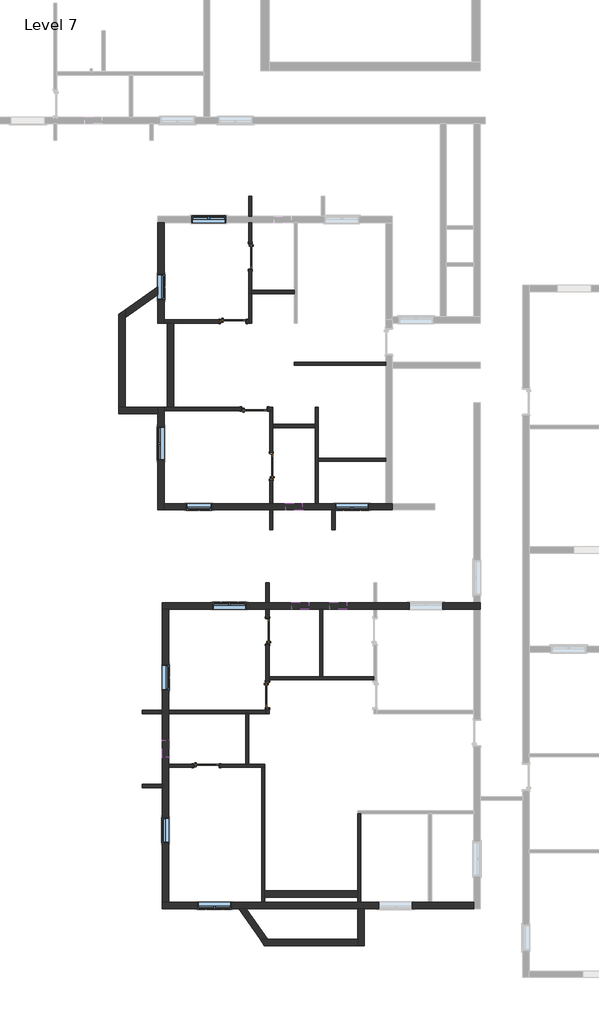
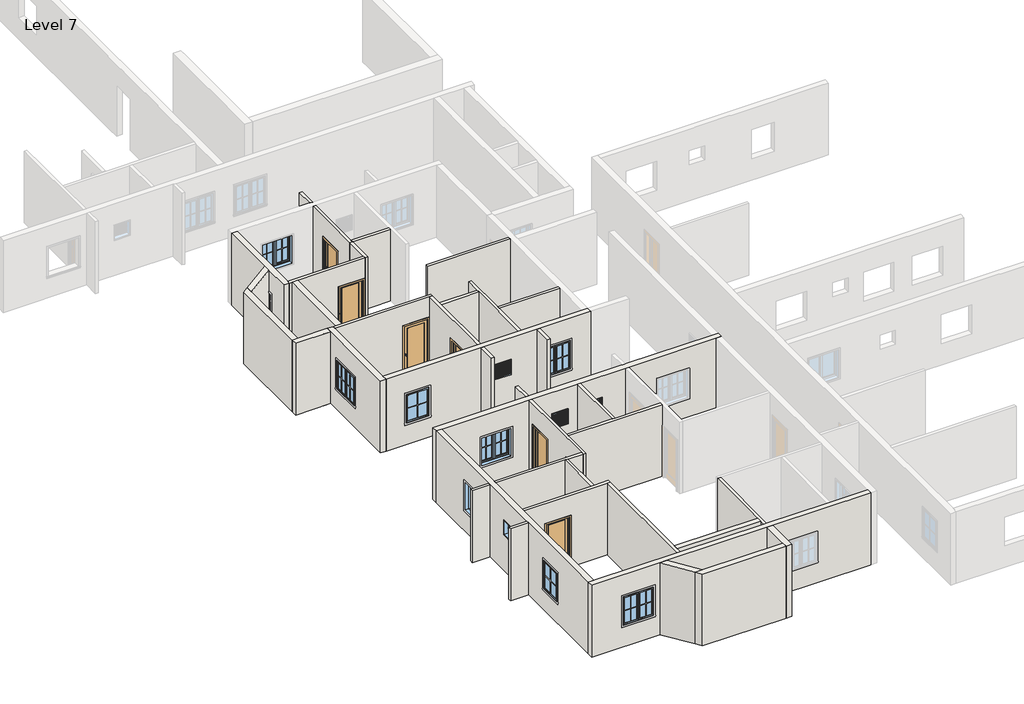
# One storey, part 1 of 7: 39 walls, 13 windows, 7 doors.
"""IFC4 building model written with IfcOpenShell, lengths in millimetres."""

from ifc_helpers import new_model, si_unit, frame, origin, place, context, project, spatial, polyline, outline, extrude, faceted_brep, transform, mapped, element, save
from components import door_3c6ab76a, door_a3feeac7, window_272f20d6, window_casement_double_4_x_4_af3140d2, window_f2d8fef0

model = new_model("IFC4")

# Units and contexts
model_context = context("Model", 3, world=origin())
ifc_project = project(units=[si_unit("LENGTHUNIT", "METRE", prefix="MILLI")], contexts=[model_context])

# Site, building, storey
site = spatial("IfcSite", under=ifc_project)
building = spatial("IfcBuilding", under=site)
storey = spatial("IfcBuildingStorey", under=building, Name="Level 7", Elevation=9601.2)

# Doors
placement = place(None, origin())
door_shape = door_3c6ab76a(model_context)
element("IfcDoor", 1, ObjectType="Door-Interior-Single-1_Panel-Wood : 2'6\" x 7' door", at=placement, inside=storey, context=model_context, shape_type="MappedRepresentation", body=[
    mapped(door_shape, transform((-4216.6759469, -3460.4538828, 9601.2), x_axis=(0.0, -1.0, 0.0), y_axis=(1.0, 0.0, 0.0), z_axis=(0.0, 0.0, 1.0))),
])
element("IfcDoor", 2, ObjectType="Door-Interior-Single-1_Panel-Wood : 2'6\" x 7' door", at=placement, inside=storey, context=model_context, shape_type="MappedRepresentation", body=[
    mapped(door_shape, transform((-5797.8259469, -21840.5288828, 9601.2), x_axis=(1.0, 0.0, 0.0), y_axis=(0.0, 1.0, 0.0), z_axis=(0.0, 0.0, 1.0))),
])
door_2_shape = door_a3feeac7(model_context)
element("IfcDoor", 3, ObjectType="Door-Interior-Single-1_Panel-Wood : 2'6\" x 7' door", at=placement, inside=storey, context=model_context, shape_type="MappedRepresentation", body=[
    mapped(door_2_shape, transform((-3454.6759469, -11032.8288828, 9601.2), x_axis=(0.0, 1.0, 0.0), y_axis=(-1.0, 0.0, 0.0), z_axis=(0.0, 0.0, 1.0))),
])
element("IfcDoor", 4, ObjectType="Door-Interior-Single-1_Panel-Wood : 2'6\" x 7' door", at=placement, inside=storey, context=model_context, shape_type="MappedRepresentation", body=[
    mapped(door_2_shape, transform((-3594.3759469, -16985.9538828, 9601.2), x_axis=(0.0, 1.0, 0.0), y_axis=(-1.0, 0.0, 0.0), z_axis=(0.0, 0.0, 1.0))),
])
element("IfcDoor", 5, ObjectType="Door-Interior-Single-1_Panel-Wood : 36\" x 84\"", at=placement, inside=storey, context=model_context, shape_type="MappedRepresentation", body=[
    mapped(door_shape, transform((-4829.4509469, -5800.4288828, 9601.2), x_axis=(1.0, 0.0, 0.0), y_axis=(0.0, 1.0, 0.0), z_axis=(0.0, 0.0, 1.0))),
])
element("IfcDoor", 6, ObjectType="Door-Interior-Single-1_Panel-Wood : 36\" x 84\"", at=placement, inside=storey, context=model_context, shape_type="MappedRepresentation", body=[
    mapped(door_2_shape, transform((-4067.4509469, -8969.0788828, 9601.2), x_axis=(1.0, 0.0, 0.0), y_axis=(0.0, 1.0, 0.0), z_axis=(0.0, 0.0, 1.0))),
])
element("IfcDoor", 7, ObjectType="Door-Interior-Single-1_Panel-Wood : 36\" x 84\"", at=placement, inside=storey, context=model_context, shape_type="MappedRepresentation", body=[
    mapped(door_2_shape, transform((-3600.7259469, -19291.0038828, 9601.2), x_axis=(0.0, -1.0, 0.0), y_axis=(1.0, 0.0, 0.0), z_axis=(0.0, 0.0, 1.0))),
])

# Walls
element("IfcWall", 8, ObjectType="4.5\" wall", at=placement, inside=storey, context=model_context, shape_type="Brep", body=[
    faceted_brep([(-4277.0009469, -4793.9538828, 12649.2), (-4277.0009469, -2241.2538828, 12649.2), (-4277.0009469, -2241.2538828, 9601.2), (-4277.0009469, -2977.8538828, 9601.2), (-4277.0009469, -2977.8538828, 11760.2), (-4277.0009469, -3943.0538828, 11760.2), (-4277.0009469, -3943.0538828, 9601.2), (-4277.0009469, -4793.9538828, 9601.2), (-4162.7009469, -2241.2538828, 12649.2), (-4162.7009469, -4679.6538828, 12649.2), (-4162.7009469, -4793.9538828, 12649.2), (-4162.7009469, -4793.9538828, 9601.2), (-4162.7009469, -4679.6538828, 9601.2), (-4162.7009469, -3943.0538828, 9601.2), (-4162.7009469, -3943.0538828, 11760.2), (-4162.7009469, -2977.8538828, 11760.2), (-4162.7009469, -2977.8538828, 9601.2), (-4162.7009469, -2241.2538828, 9601.2)], [[[0, 1, 2, 3, 4, 5, 6, 7]], [[8, 9, 10, 11, 12, 13, 14, 15, 16, 17]], [[2, 17, 16, 3]], [[11, 7, 6, 13, 12]], [[1, 0, 10, 9, 8]], [[2, 1, 8, 17]], [[0, 7, 11, 10]], [[5, 14, 13, 6]], [[14, 5, 4, 15]], [[15, 4, 3, 16]]]),
])
element("IfcWall", 9, ObjectType="4.5\" wall", at=placement, inside=storey, context=model_context, shape_type="Brep", body=[
    faceted_brep([(-4277.0009469, -4793.9538828, 9601.2), (-4277.0009469, -5746.4538828, 9601.2), (-4277.0009469, -5860.7538828, 9601.2), (-4277.0009469, -5860.7538828, 12649.2), (-4277.0009469, -5746.4538828, 12649.2), (-4277.0009469, -4793.9538828, 12649.2), (-4162.7009469, -4793.9538828, 9601.2), (-4162.7009469, -4793.9538828, 12649.2), (-4162.7009469, -5860.7538828, 12649.2), (-4162.7009469, -5860.7538828, 9601.2)], [[[0, 1, 2, 3, 4, 5]], [[6, 7, 8, 9]], [[2, 1, 0, 6, 9]], [[5, 4, 3, 8, 7]], [[0, 5, 7, 6]], [[3, 2, 9, 8]]]),
])
element("IfcWall", 10, ObjectType="4.5\" wall", at=placement, inside=storey, context=model_context, shape_type="Brep", body=[
    faceted_brep([(-7325.0009469, -5746.4538828, 12649.2), (-4277.0009469, -5746.4538828, 12649.2), (-4277.0009469, -5746.4538828, 9601.2), (-4346.8509469, -5746.4538828, 9601.2), (-4346.8509469, -5746.4538828, 11760.2), (-5312.0509469, -5746.4538828, 11760.2), (-5312.0509469, -5746.4538828, 9601.2), (-7325.0009469, -5746.4538828, 9601.2), (-4277.0009469, -5860.7538828, 12649.2), (-6982.1009469, -5860.7538828, 12649.2), (-7210.7009469, -5860.7538828, 12649.2), (-7325.0009469, -5860.7538828, 12649.2), (-7325.0009469, -5860.7538828, 9601.2), (-7210.7009469, -5860.7538828, 9601.2), (-6982.1009469, -5860.7538828, 9601.2), (-5312.0509469, -5860.7538828, 9601.2), (-5312.0509469, -5860.7538828, 11760.2), (-4346.8509469, -5860.7538828, 11760.2), (-4346.8509469, -5860.7538828, 9601.2), (-4277.0009469, -5860.7538828, 9601.2)], [[[0, 1, 2, 3, 4, 5, 6, 7]], [[8, 9, 10, 11, 12, 13, 14, 15, 16, 17, 18, 19]], [[12, 7, 6, 15, 14, 13]], [[2, 19, 18, 3]], [[1, 0, 11, 10, 9, 8]], [[0, 7, 12, 11]], [[2, 1, 8, 19]], [[17, 4, 3, 18]], [[4, 17, 16, 5]], [[5, 16, 15, 6]]]),
])
element("IfcWall", 11, ObjectType="4.5\" wall", at=placement, inside=storey, context=model_context, shape_type="SweptSolid", body=[
    extrude(outline(polyline([(-2638.7009469, -4793.9538828), (-4162.7009469, -4793.9538828), (-4162.7009469, -4679.6538828), (-2638.7009469, -4679.6538828), (-2638.7009469, -4793.9538828)])), frame((0.0, 0.0, 9601.2), z_axis=(0.0, 0.0, 1.0), x_axis=(1.0, 0.0, 0.0)), (0.0, 0.0, 1.0), 3048.0),
])
element("IfcWall", 12, ObjectType="4.5\" wall", at=placement, inside=storey, context=model_context, shape_type="SweptSolid", body=[
    extrude(outline(polyline([(-2638.7009469, -7270.4538828), (675.9990531, -7270.4538828), (675.9990531, -7384.7538828), (-2638.7009469, -7384.7538828), (-2638.7009469, -7270.4538828)])), frame((0.0, 0.0, 9601.2), z_axis=(0.0, 0.0, 1.0), x_axis=(1.0, 0.0, 0.0)), (0.0, 0.0, 1.0), 3048.0),
])
element("IfcWall", 13, ObjectType="4.5\" wall", at=placement, inside=storey, context=model_context, shape_type="Brep", body=[
    faceted_brep([(-7325.0009469, -8908.7538828, 12649.2), (-7210.7009469, -8908.7538828, 12649.2), (-6982.1009469, -8908.7538828, 12649.2), (-3400.7009469, -8908.7538828, 12649.2), (-3400.7009469, -8908.7538828, 9601.2), (-3584.8509469, -8908.7538828, 9601.2), (-3584.8509469, -8908.7538828, 11760.2), (-4550.0509469, -8908.7538828, 11760.2), (-4550.0509469, -8908.7538828, 9601.2), (-6982.1009469, -8908.7538828, 9601.2), (-7210.7009469, -8908.7538828, 9601.2), (-7325.0009469, -8908.7538828, 9601.2), (-3400.7009469, -9023.0538828, 12649.2), (-3515.0009469, -9023.0538828, 12649.2), (-7325.0009469, -9023.0538828, 12649.2), (-7325.0009469, -9023.0538828, 9601.2), (-4550.0509469, -9023.0538828, 9601.2), (-4550.0509469, -9023.0538828, 11760.2), (-3584.8509469, -9023.0538828, 11760.2), (-3584.8509469, -9023.0538828, 9601.2), (-3515.0009469, -9023.0538828, 9601.2), (-3400.7009469, -9023.0538828, 9601.2)], [[[0, 1, 2, 3, 4, 5, 6, 7, 8, 9, 10, 11]], [[12, 13, 14, 15, 16, 17, 18, 19, 20, 21]], [[4, 21, 20, 19, 5]], [[15, 11, 10, 9, 8, 16]], [[3, 2, 1, 0, 14, 13, 12]], [[4, 3, 12, 21]], [[0, 11, 15, 14]], [[18, 6, 5, 19]], [[6, 18, 17, 7]], [[7, 17, 16, 8]]]),
])
element("IfcWall", 14, ObjectType="4.5\" wall", at=placement, inside=storey, context=model_context, shape_type="SweptSolid", body=[
    extrude(outline(polyline([(-1876.7009469, -9632.6538828), (-3400.7009469, -9632.6538828), (-3400.7009469, -9518.3538828), (-1876.7009469, -9518.3538828), (-1876.7009469, -9632.6538828)])), frame((0.0, 0.0, 9601.2), z_axis=(0.0, 0.0, 1.0), x_axis=(1.0, 0.0, 0.0)), (0.0, 0.0, 1.0), 3048.0),
])
element("IfcWall", 15, ObjectType="4.5\" wall", at=placement, inside=storey, context=model_context, shape_type="Brep", body=[
    faceted_brep([(-1762.4009469, -12375.8538828, 9601.2), (-1762.4009469, -10851.8538828, 9601.2), (-1762.4009469, -10737.5538828, 9601.2), (-1762.4009469, -8908.7538828, 9601.2), (-1762.4009469, -8908.7538828, 12649.2), (-1762.4009469, -10737.5538828, 12649.2), (-1762.4009469, -10851.8538828, 12649.2), (-1762.4009469, -12375.8538828, 12649.2), (-1876.7009469, -12375.8538828, 9601.2), (-1876.7009469, -12375.8538828, 12649.2), (-1876.7009469, -9632.6538828, 12649.2), (-1876.7009469, -9518.3538828, 12649.2), (-1876.7009469, -8908.7538828, 12649.2), (-1876.7009469, -8908.7538828, 9601.2), (-1876.7009469, -9518.3538828, 9601.2), (-1876.7009469, -9632.6538828, 9601.2)], [[[0, 1, 2, 3, 4, 5, 6, 7]], [[8, 9, 10, 11, 12, 13, 14, 15]], [[3, 2, 1, 0, 8, 15, 14, 13]], [[4, 3, 13, 12]], [[7, 6, 5, 4, 12, 11, 10, 9]], [[0, 7, 9, 8]]]),
])
element("IfcWall", 16, ObjectType="4.5\" wall", at=placement, inside=storey, context=model_context, shape_type="Brep", body=[
    faceted_brep([(-3400.7009469, -9023.0538828, 12649.2), (-3400.7009469, -9518.3538828, 12649.2), (-3400.7009469, -9632.6538828, 12649.2), (-3400.7009469, -12375.8538828, 12649.2), (-3400.7009469, -12375.8538828, 9601.2), (-3400.7009469, -11515.4288828, 9601.2), (-3400.7009469, -11515.4288828, 11760.2), (-3400.7009469, -10550.2288828, 11760.2), (-3400.7009469, -10550.2288828, 9601.2), (-3400.7009469, -9632.6538828, 9601.2), (-3400.7009469, -9518.3538828, 9601.2), (-3400.7009469, -9023.0538828, 9601.2), (-3515.0009469, -12375.8538828, 12649.2), (-3515.0009469, -9023.0538828, 12649.2), (-3515.0009469, -9023.0538828, 9601.2), (-3515.0009469, -10550.2288828, 9601.2), (-3515.0009469, -10550.2288828, 11760.2), (-3515.0009469, -11515.4288828, 11760.2), (-3515.0009469, -11515.4288828, 9601.2), (-3515.0009469, -12375.8538828, 9601.2)], [[[0, 1, 2, 3, 4, 5, 6, 7, 8, 9, 10, 11]], [[12, 13, 14, 15, 16, 17, 18, 19]], [[4, 19, 18, 5]], [[14, 11, 10, 9, 8, 15]], [[3, 2, 1, 0, 13, 12]], [[4, 3, 12, 19]], [[0, 11, 14, 13]], [[7, 16, 15, 8]], [[16, 7, 6, 17]], [[17, 6, 5, 18]]]),
])
element("IfcWall", 17, ObjectType="4.5\" wall", at=placement, inside=storey, context=model_context, shape_type="SweptSolid", body=[
    extrude(outline(polyline([(-1762.4009469, -10737.5538828), (675.9990531, -10737.5538828), (675.9990531, -10851.8538828), (-1762.4009469, -10851.8538828), (-1762.4009469, -10737.5538828)])), frame((0.0, 0.0, 9601.2), z_axis=(0.0, 0.0, 1.0), x_axis=(1.0, 0.0, 0.0)), (0.0, 0.0, 1.0), 3048.0),
])
element("IfcWall", 18, ObjectType="4.5\" wall", at=placement, inside=storey, context=model_context, shape_type="SweptSolid", body=[
    extrude(outline(polyline([(-3515.0009469, -13328.3538828), (-3515.0009469, -12604.4538828), (-3400.7009469, -12604.4538828), (-3400.7009469, -13328.3538828), (-3515.0009469, -13328.3538828)])), frame((0.0, 0.0, 9601.2), z_axis=(0.0, 0.0, 1.0), x_axis=(1.0, 0.0, 0.0)), (0.0, 0.0, 1.0), 3048.0),
])
element("IfcWall", 19, ObjectType="4.5\" wall", at=placement, inside=storey, context=model_context, shape_type="Brep", body=[
    faceted_brep([(-1152.8009469, -13328.3538828, 9601.2), (-1152.8009469, -12604.4538828, 9601.2), (-1152.8009469, -12604.4538828, 10515.6), (-1152.8009469, -12604.4538828, 11734.8), (-1152.8009469, -12604.4538828, 12649.2), (-1152.8009469, -13328.3538828, 12649.2), (-1267.1009469, -13328.3538828, 9601.2), (-1267.1009469, -13328.3538828, 12649.2), (-1267.1009469, -12604.4538828, 12649.2), (-1267.1009469, -12604.4538828, 9601.2)], [[[0, 1, 2, 3, 4, 5]], [[6, 7, 8, 9]], [[1, 0, 6, 9]], [[5, 4, 8, 7]], [[0, 5, 7, 6]], [[4, 3, 2, 1, 9, 8]]]),
])
element("IfcWall", 20, ObjectType="4.5\" wall", at=placement, inside=storey, context=model_context, shape_type="SweptSolid", body=[
    extrude(outline(polyline([(-4162.7009469, -1288.7538828), (-4162.7009469, -2012.6538828), (-4277.0009469, -2012.6538828), (-4277.0009469, -1288.7538828), (-4162.7009469, -1288.7538828)])), frame((0.0, 0.0, 9601.2), z_axis=(0.0, 0.0, 1.0), x_axis=(1.0, 0.0, 0.0)), (0.0, 0.0, 1.0), 3048.0),
])
element("IfcWall", 21, ObjectType="4.5\" wall", at=placement, inside=storey, context=model_context, shape_type="Brep", body=[
    faceted_brep([(231.4990531, -18624.2538828, 9601.2), (-1597.3009469, -18624.2538828, 9601.2), (-1711.6009469, -18624.2538828, 9601.2), (-3540.4009469, -18624.2538828, 9601.2), (-3540.4009469, -18624.2538828, 12649.2), (-1711.6009469, -18624.2538828, 12649.2), (-1597.3009469, -18624.2538828, 12649.2), (231.4990531, -18624.2538828, 12649.2), (231.4990531, -18738.5538828, 9601.2), (231.4990531, -18738.5538828, 12649.2), (-3540.4009469, -18738.5538828, 12649.2), (-3540.4009469, -18738.5538828, 9601.2)], [[[0, 1, 2, 3, 4, 5, 6, 7]], [[8, 9, 10, 11]], [[3, 2, 1, 0, 8, 11]], [[7, 6, 5, 4, 10, 9]], [[4, 3, 11, 10]], [[0, 7, 9, 8]]]),
])
element("IfcWall", 22, ObjectType="4.5\" wall", at=placement, inside=storey, context=model_context, shape_type="SweptSolid", body=[
    extrude(outline(polyline([(-1597.3009469, -16185.8538828), (-1597.3009469, -18624.2538828), (-1711.6009469, -18624.2538828), (-1711.6009469, -16185.8538828), (-1597.3009469, -16185.8538828)])), frame((0.0, 0.0, 9601.2), z_axis=(0.0, 0.0, 1.0), x_axis=(1.0, 0.0, 0.0)), (0.0, 0.0, 1.0), 3048.0),
])
element("IfcWall", 23, ObjectType="4.5\" wall", at=placement, inside=storey, context=model_context, shape_type="SweptSolid", body=[
    extrude(outline(polyline([(-3540.4009469, -15233.3538828), (-3540.4009469, -15957.2538828), (-3654.7009469, -15957.2538828), (-3654.7009469, -15233.3538828), (-3540.4009469, -15233.3538828)])), frame((0.0, 0.0, 9601.2), z_axis=(0.0, 0.0, 1.0), x_axis=(1.0, 0.0, 0.0)), (0.0, 0.0, 1.0), 3048.0),
])
element("IfcWall", 24, ObjectType="4.5\" wall", at=placement, inside=storey, context=model_context, shape_type="Brep", body=[
    faceted_brep([(-3654.7009469, -19957.7538828, 12649.2), (-3654.7009469, -19843.4538828, 12649.2), (-3654.7009469, -16185.8538828, 12649.2), (-3654.7009469, -16185.8538828, 9601.2), (-3654.7009469, -16503.3538828, 9601.2), (-3654.7009469, -16503.3538828, 11760.2), (-3654.7009469, -17468.5538828, 11760.2), (-3654.7009469, -17468.5538828, 9601.2), (-3654.7009469, -18808.4038828, 9601.2), (-3654.7009469, -18808.4038828, 11760.2), (-3654.7009469, -19773.6038828, 11760.2), (-3654.7009469, -19773.6038828, 9601.2), (-3654.7009469, -19843.4538828, 9601.2), (-3654.7009469, -19957.7538828, 9601.2), (-3540.4009469, -16185.8538828, 12649.2), (-3540.4009469, -18624.2538828, 12649.2), (-3540.4009469, -18738.5538828, 12649.2), (-3540.4009469, -19957.7538828, 12649.2), (-3540.4009469, -19957.7538828, 9601.2), (-3540.4009469, -19773.6038828, 9601.2), (-3540.4009469, -19773.6038828, 11760.2), (-3540.4009469, -18808.4038828, 11760.2), (-3540.4009469, -18808.4038828, 9601.2), (-3540.4009469, -18738.5538828, 9601.2), (-3540.4009469, -18624.2538828, 9601.2), (-3540.4009469, -17468.5538828, 9601.2), (-3540.4009469, -17468.5538828, 11760.2), (-3540.4009469, -16503.3538828, 11760.2), (-3540.4009469, -16503.3538828, 9601.2), (-3540.4009469, -16185.8538828, 9601.2)], [[[0, 1, 2, 3, 4, 5, 6, 7, 8, 9, 10, 11, 12, 13]], [[14, 15, 16, 17, 18, 19, 20, 21, 22, 23, 24, 25, 26, 27, 28, 29]], [[3, 29, 28, 4]], [[18, 13, 12, 11, 19]], [[7, 25, 24, 23, 22, 8]], [[2, 1, 0, 17, 16, 15, 14]], [[3, 2, 14, 29]], [[0, 13, 18, 17]], [[27, 5, 4, 28]], [[5, 27, 26, 6]], [[6, 26, 25, 7]], [[10, 20, 19, 11]], [[20, 10, 9, 21]], [[21, 9, 8, 22]]]),
])
element("IfcWall", 25, ObjectType="4.5\" wall", at=placement, inside=storey, context=model_context, shape_type="Brep", body=[
    faceted_brep([(-3654.7009469, -19843.4538828, 9601.2), (-7159.9009469, -19843.4538828, 9601.2), (-7159.9009469, -19843.4538828, 12649.2), (-3654.7009469, -19843.4538828, 12649.2), (-3654.7009469, -19957.7538828, 9601.2), (-3654.7009469, -19957.7538828, 12649.2), (-4264.3009469, -19957.7538828, 12649.2), (-4378.6009469, -19957.7538828, 12649.2), (-7159.9009469, -19957.7538828, 12649.2), (-7159.9009469, -19957.7538828, 9601.2), (-4378.6009469, -19957.7538828, 9601.2), (-4264.3009469, -19957.7538828, 9601.2)], [[[0, 1, 2, 3]], [[4, 5, 6, 7, 8, 9, 10, 11]], [[1, 0, 4, 11, 10, 9]], [[3, 2, 8, 7, 6, 5]], [[2, 1, 9, 8]], [[0, 3, 5, 4]]]),
])
element("IfcWall", 26, ObjectType="4.5\" wall", at=placement, inside=storey, context=model_context, shape_type="Brep", body=[
    faceted_brep([(-7159.9009469, -21786.5538828, 12649.2), (-4378.6009469, -21786.5538828, 12649.2), (-4264.3009469, -21786.5538828, 12649.2), (-3692.8009469, -21786.5538828, 12649.2), (-3692.8009469, -21786.5538828, 9601.2), (-4264.3009469, -21786.5538828, 9601.2), (-4378.6009469, -21786.5538828, 9601.2), (-5315.2259469, -21786.5538828, 9601.2), (-5315.2259469, -21786.5538828, 11760.2), (-6280.4259469, -21786.5538828, 11760.2), (-6280.4259469, -21786.5538828, 9601.2), (-7159.9009469, -21786.5538828, 9601.2), (-3692.8009469, -21900.8538828, 12649.2), (-3807.1009469, -21900.8538828, 12649.2), (-7159.9009469, -21900.8538828, 12649.2), (-7159.9009469, -21900.8538828, 9601.2), (-6280.4259469, -21900.8538828, 9601.2), (-6280.4259469, -21900.8538828, 11760.2), (-5315.2259469, -21900.8538828, 11760.2), (-5315.2259469, -21900.8538828, 9601.2), (-3807.1009469, -21900.8538828, 9601.2), (-3692.8009469, -21900.8538828, 9601.2)], [[[0, 1, 2, 3, 4, 5, 6, 7, 8, 9, 10, 11]], [[12, 13, 14, 15, 16, 17, 18, 19, 20, 21]], [[15, 11, 10, 16]], [[4, 21, 20, 19, 7, 6, 5]], [[3, 2, 1, 0, 14, 13, 12]], [[0, 11, 15, 14]], [[4, 3, 12, 21]], [[18, 8, 7, 19]], [[8, 18, 17, 9]], [[9, 17, 16, 10]]]),
])
element("IfcWall", 27, ObjectType="4.5\" wall", at=placement, inside=storey, context=model_context, shape_type="Brep", body=[
    faceted_brep([(-3692.8009469, -26777.6538828, 9601.2), (-3692.8009469, -26587.1538828, 9601.2), (-3692.8009469, -26358.5538828, 9601.2), (-3692.8009469, -21900.8538828, 9601.2), (-3692.8009469, -21900.8538828, 12649.2), (-3692.8009469, -26358.5538828, 12649.2), (-3692.8009469, -26587.1538828, 12649.2), (-3692.8009469, -26777.6538828, 12649.2), (-3807.1009469, -26777.6538828, 9601.2), (-3807.1009469, -26777.6538828, 12649.2), (-3807.1009469, -21900.8538828, 12649.2), (-3807.1009469, -21900.8538828, 9601.2)], [[[0, 1, 2, 3, 4, 5, 6, 7]], [[8, 9, 10, 11]], [[3, 2, 1, 0, 8, 11]], [[7, 6, 5, 4, 10, 9]], [[4, 3, 11, 10]], [[0, 7, 9, 8]]]),
])
element("IfcWall", 28, ObjectType="4.5\" wall", at=placement, inside=storey, context=model_context, shape_type="SweptSolid", body=[
    extrude(outline(polyline([(-7388.5009469, -22629.8863256), (-8112.4009469, -22629.8863256), (-8112.4009469, -22515.5863256), (-7388.5009469, -22515.5863256), (-7388.5009469, -22629.8863256)])), frame((0.0, 0.0, 9601.2), z_axis=(0.0, 0.0, 1.0), x_axis=(1.0, 0.0, 0.0)), (0.0, 0.0, 1.0), 3048.0),
])
element("IfcWall", 29, ObjectType="4.5\" wall", at=placement, inside=storey, context=model_context, shape_type="SweptSolid", body=[
    extrude(outline(polyline([(-8112.4009469, -19843.4538828), (-7388.5009469, -19843.4538828), (-7388.5009469, -19957.7538828), (-8112.4009469, -19957.7538828), (-8112.4009469, -19843.4538828)])), frame((0.0, 0.0, 9601.2), z_axis=(0.0, 0.0, 1.0), x_axis=(1.0, 0.0, 0.0)), (0.0, 0.0, 1.0), 3048.0),
])
element("IfcWall", 30, ObjectType="4.5\" wall", at=placement, inside=storey, context=model_context, shape_type="SweptSolid", body=[
    extrude(outline(polyline([(-4378.6009469, -21786.5538828), (-4378.6009469, -19957.7538828), (-4264.3009469, -19957.7538828), (-4264.3009469, -21786.5538828), (-4378.6009469, -21786.5538828)])), frame((0.0, 0.0, 9601.2), z_axis=(0.0, 0.0, 1.0), x_axis=(1.0, 0.0, 0.0)), (0.0, 0.0, 1.0), 3048.0),
])
element("IfcWall", 31, ObjectType="4.5\" wall", at=placement, inside=storey, context=model_context, shape_type="Brep", body=[
    faceted_brep([(-340.0009469, -23577.2538828, 9601.2), (-340.0009469, -26358.5538828, 9601.2), (-340.0009469, -26587.1538828, 9601.2), (-340.0009469, -26777.6538828, 9601.2), (-340.0009469, -26777.6538828, 12649.2), (-340.0009469, -26587.1538828, 12649.2), (-340.0009469, -26358.5538828, 12649.2), (-340.0009469, -23577.2538828, 12649.2), (-225.7009469, -23577.2538828, 9601.2), (-225.7009469, -23577.2538828, 12649.2), (-225.7009469, -26777.6538828, 12649.2), (-225.7009469, -26777.6538828, 9601.2)], [[[0, 1, 2, 3, 4, 5, 6, 7]], [[8, 9, 10, 11]], [[3, 2, 1, 0, 8, 11]], [[7, 6, 5, 4, 10, 9]], [[0, 7, 9, 8]], [[4, 3, 11, 10]]]),
])
element("IfcWall", 32, ObjectType="9\"", at=placement, inside=storey, context=model_context, shape_type="Brep", body=[
    faceted_brep([(-7553.6009469, -2241.2538828, 9601.2), (-7553.6009469, -4556.8220214, 9601.2), (-7553.6009469, -4835.8638828, 9601.2), (-7553.6009469, -5860.7538828, 9601.2), (-7553.6009469, -5860.7538828, 12649.2), (-7553.6009469, -4835.8638828, 12649.2), (-7553.6009469, -4556.8220214, 12649.2), (-7553.6009469, -2241.2538828, 12649.2), (-7553.6009469, -5016.2038828, 11734.8), (-7553.6009469, -5016.2038828, 10515.6), (-7553.6009469, -4101.8038828, 10515.6), (-7553.6009469, -4101.8038828, 11734.8), (-7325.0009469, -2241.2538828, 9601.2), (-7325.0009469, -2241.2538828, 12649.2), (-7325.0009469, -5746.4538828, 12649.2), (-7325.0009469, -5860.7538828, 12649.2), (-7325.0009469, -5860.7538828, 9601.2), (-7325.0009469, -5746.4538828, 9601.2), (-7325.0009469, -5016.2038828, 11734.8), (-7325.0009469, -4101.8038828, 11734.8), (-7325.0009469, -4101.8038828, 10515.6), (-7325.0009469, -5016.2038828, 10515.6)], [[[0, 1, 2, 3, 4, 5, 6, 7], [8, 9, 10, 11]], [[12, 13, 14, 15, 16, 17], [18, 19, 20, 21]], [[3, 2, 1, 0, 12, 17, 16]], [[7, 6, 5, 4, 15, 14, 13]], [[0, 7, 13, 12]], [[4, 3, 16, 15]], [[9, 8, 18, 21]], [[10, 9, 21, 20]], [[11, 10, 20, 19]], [[8, 11, 19, 18]]]),
])
element("IfcWall", 33, ObjectType="9\"", at=placement, inside=storey, context=model_context, shape_type="SweptSolid", body=[
    extrude(outline(polyline([(-6982.1009469, -5860.7538828), (-6982.1009469, -8908.7538828), (-7210.7009469, -8908.7538828), (-7210.7009469, -5860.7538828), (-6982.1009469, -5860.7538828)])), frame((0.0, 0.0, 9601.2), z_axis=(0.0, 0.0, 1.0), x_axis=(1.0, 0.0, 0.0)), (0.0, 0.0, 1.0), 3048.0),
])
element("IfcWall", 34, ObjectType="9\"", at=placement, inside=storey, context=model_context, shape_type="Brep", body=[
    faceted_brep([(-7553.6009469, -8908.7538828, 9601.2), (-7553.6009469, -9137.3538828, 9601.2), (-7553.6009469, -12604.4538828, 9601.2), (-7553.6009469, -12604.4538828, 12649.2), (-7553.6009469, -9137.3538828, 12649.2), (-7553.6009469, -8908.7538828, 12649.2), (-7553.6009469, -9600.9038828, 11734.8), (-7553.6009469, -10820.1038828, 11734.8), (-7553.6009469, -10820.1038828, 10515.6), (-7553.6009469, -9600.9038828, 10515.6), (-7325.0009469, -8908.7538828, 9601.2), (-7325.0009469, -8908.7538828, 12649.2), (-7325.0009469, -9023.0538828, 12649.2), (-7325.0009469, -12375.8538828, 12649.2), (-7325.0009469, -12604.4538828, 12649.2), (-7325.0009469, -12604.4538828, 9601.2), (-7325.0009469, -12375.8538828, 9601.2), (-7325.0009469, -9023.0538828, 9601.2), (-7325.0009469, -9600.9038828, 11734.8), (-7325.0009469, -9600.9038828, 10515.6), (-7325.0009469, -10820.1038828, 10515.6), (-7325.0009469, -10820.1038828, 11734.8)], [[[0, 1, 2, 3, 4, 5], [6, 7, 8, 9]], [[10, 11, 12, 13, 14, 15, 16, 17], [18, 19, 20, 21]], [[2, 1, 0, 10, 17, 16, 15]], [[5, 4, 3, 14, 13, 12, 11]], [[3, 2, 15, 14]], [[0, 5, 11, 10]], [[19, 18, 6, 9]], [[20, 19, 9, 8]], [[21, 20, 8, 7]], [[18, 21, 7, 6]]]),
])
element("IfcWall", 35, ObjectType="9\"", at=placement, inside=storey, context=model_context, shape_type="Brep", body=[
    faceted_brep([(-7325.0009469, -12604.4538828, 9601.2), (-3515.0009469, -12604.4538828, 9601.2), (-3400.7009469, -12604.4538828, 9601.2), (-1267.1009469, -12604.4538828, 9601.2), (-1152.8009469, -12604.4538828, 9601.2), (904.5990531, -12604.4538828, 9601.2), (904.5990531, -12604.4538828, 12649.2), (-1152.8009469, -12604.4538828, 12649.2), (-1267.1009469, -12604.4538828, 12649.2), (-3400.7009469, -12604.4538828, 12649.2), (-3515.0009469, -12604.4538828, 12649.2), (-7325.0009469, -12604.4538828, 12649.2), (-2333.9009469, -12604.4538828, 11734.8), (-2333.9009469, -12604.4538828, 11125.2), (-2943.5009469, -12604.4538828, 11125.2), (-2943.5009469, -12604.4538828, 11734.8), (-6524.9009469, -12604.4538828, 11734.8), (-5610.5009469, -12604.4538828, 11734.8), (-5610.5009469, -12604.4538828, 10515.6), (-6524.9009469, -12604.4538828, 10515.6), (-1152.8009469, -12604.4538828, 11734.8), (66.3990531, -12604.4538828, 11734.8), (66.3990531, -12604.4538828, 10515.6), (-1152.8009469, -12604.4538828, 10515.6), (-7325.0009469, -12375.8538828, 9601.2), (-7325.0009469, -12375.8538828, 12649.2), (-3515.0009469, -12375.8538828, 12649.2), (-3400.7009469, -12375.8538828, 12649.2), (-1876.7009469, -12375.8538828, 12649.2), (-1762.4009469, -12375.8538828, 12649.2), (675.9990531, -12375.8538828, 12649.2), (904.5990531, -12375.8538828, 12649.2), (904.5990531, -12375.8538828, 9601.2), (675.9990531, -12375.8538828, 9601.2), (-1762.4009469, -12375.8538828, 9601.2), (-1876.7009469, -12375.8538828, 9601.2), (-3400.7009469, -12375.8538828, 9601.2), (-3515.0009469, -12375.8538828, 9601.2), (-2333.9009469, -12375.8538828, 11734.8), (-2943.5009469, -12375.8538828, 11734.8), (-2943.5009469, -12375.8538828, 11125.2), (-2333.9009469, -12375.8538828, 11125.2), (-6524.9009469, -12375.8538828, 11734.8), (-6524.9009469, -12375.8538828, 10515.6), (-5610.5009469, -12375.8538828, 10515.6), (-5610.5009469, -12375.8538828, 11734.8), (-1152.8009469, -12375.8538828, 11734.8), (-1152.8009469, -12375.8538828, 10515.6), (66.3990531, -12375.8538828, 10515.6), (66.3990531, -12375.8538828, 11734.8)], [[[0, 1, 2, 3, 4, 5, 6, 7, 8, 9, 10, 11], [12, 13, 14, 15], [16, 17, 18, 19], [20, 21, 22, 23]], [[24, 25, 26, 27, 28, 29, 30, 31, 32, 33, 34, 35, 36, 37], [38, 39, 40, 41], [42, 43, 44, 45], [46, 47, 48, 49]], [[5, 4, 3, 2, 1, 0, 24, 37, 36, 35, 34, 33, 32]], [[11, 10, 9, 8, 7, 6, 31, 30, 29, 28, 27, 26, 25]], [[0, 11, 25, 24]], [[6, 5, 32, 31]], [[13, 12, 38, 41]], [[14, 13, 41, 40]], [[15, 14, 40, 39]], [[12, 15, 39, 38]], [[43, 42, 16, 19]], [[44, 43, 19, 18]], [[45, 44, 18, 17]], [[42, 45, 17, 16]], [[47, 46, 20, 23]], [[48, 47, 23, 22]], [[49, 48, 22, 21]], [[46, 49, 21, 20]]]),
])
element("IfcWall", 36, ObjectType="9\"", at=placement, inside=storey, context=model_context, shape_type="SweptSolid", body=[
    extrude(outline(polyline([(-7820.3009469, -8908.7538828), (-7553.6009469, -8908.7538828), (-7553.6009469, -9137.3538828), (-7820.3009469, -9137.3538828), (-7820.3009469, -8908.7538828)])), frame((0.0, 0.0, 9601.2), z_axis=(0.0, 0.0, 1.0), x_axis=(1.0, 0.0, 0.0)), (0.0, 0.0, 1.0), 3048.0),
])
element("IfcWall", 37, ObjectType="9\"", at=placement, inside=storey, context=model_context, shape_type="Brep", body=[
    faceted_brep([(-7388.5009469, -16185.8538828, 9601.2), (-7159.9009469, -16185.8538828, 9601.2), (-3654.7009469, -16185.8538828, 9601.2), (-3540.4009469, -16185.8538828, 9601.2), (-1711.6009469, -16185.8538828, 9601.2), (-1597.3009469, -16185.8538828, 9601.2), (231.4990531, -16185.8538828, 9601.2), (345.7990531, -16185.8538828, 9601.2), (3850.9990531, -16185.8538828, 9601.2), (4079.5990531, -16185.8538828, 9601.2), (4079.5990531, -16185.8538828, 12649.2), (3850.9990531, -16185.8538828, 12649.2), (345.7990531, -16185.8538828, 12649.2), (231.4990531, -16185.8538828, 12649.2), (-1597.3009469, -16185.8538828, 12649.2), (-1711.6009469, -16185.8538828, 12649.2), (-3540.4009469, -16185.8538828, 12649.2), (-3654.7009469, -16185.8538828, 12649.2), (-7159.9009469, -16185.8538828, 12649.2), (-7388.5009469, -16185.8538828, 12649.2), (-740.0509469, -16185.8538828, 11734.8), (-740.0509469, -16185.8538828, 11125.2), (-1349.6509469, -16185.8538828, 11125.2), (-1349.6509469, -16185.8538828, 11734.8), (-2111.6509469, -16185.8538828, 11734.8), (-2111.6509469, -16185.8538828, 11125.2), (-2721.2509469, -16185.8538828, 11125.2), (-2721.2509469, -16185.8538828, 11734.8), (2736.5740531, -16185.8538828, 11734.8), (2736.5740531, -16185.8538828, 10515.6), (1517.3740531, -16185.8538828, 10515.6), (1517.3740531, -16185.8538828, 11734.8), (-4359.5509469, -16185.8538828, 11734.8), (-4359.5509469, -16185.8538828, 10515.6), (-5578.7509469, -16185.8538828, 10515.6), (-5578.7509469, -16185.8538828, 11734.8), (-7388.5009469, -15957.2538828, 9601.2), (-7388.5009469, -15957.2538828, 12649.2), (-3654.7009469, -15957.2538828, 12649.2), (-3540.4009469, -15957.2538828, 12649.2), (231.4990531, -15957.2538828, 12649.2), (345.7990531, -15957.2538828, 12649.2), (3850.9990531, -15957.2538828, 12649.2), (4079.5990531, -15957.2538828, 12649.2), (4079.5990531, -15957.2538828, 9601.2), (3850.9990531, -15957.2538828, 9601.2), (345.7990531, -15957.2538828, 9601.2), (231.4990531, -15957.2538828, 9601.2), (-3540.4009469, -15957.2538828, 9601.2), (-3654.7009469, -15957.2538828, 9601.2), (-740.0509469, -15957.2538828, 11734.8), (-1349.6509469, -15957.2538828, 11734.8), (-1349.6509469, -15957.2538828, 11125.2), (-740.0509469, -15957.2538828, 11125.2), (-2111.6509469, -15957.2538828, 11734.8), (-2721.2509469, -15957.2538828, 11734.8), (-2721.2509469, -15957.2538828, 11125.2), (-2111.6509469, -15957.2538828, 11125.2), (2736.5740531, -15957.2538828, 11734.8), (1517.3740531, -15957.2538828, 11734.8), (1517.3740531, -15957.2538828, 10515.6), (2736.5740531, -15957.2538828, 10515.6), (-4359.5509469, -15957.2538828, 11734.8), (-5578.7509469, -15957.2538828, 11734.8), (-5578.7509469, -15957.2538828, 10515.6), (-4359.5509469, -15957.2538828, 10515.6)], [[[0, 1, 2, 3, 4, 5, 6, 7, 8, 9, 10, 11, 12, 13, 14, 15, 16, 17, 18, 19], [20, 21, 22, 23], [24, 25, 26, 27], [28, 29, 30, 31], [32, 33, 34, 35]], [[36, 37, 38, 39, 40, 41, 42, 43, 44, 45, 46, 47, 48, 49], [50, 51, 52, 53], [54, 55, 56, 57], [58, 59, 60, 61], [62, 63, 64, 65]], [[9, 8, 7, 6, 5, 4, 3, 2, 1, 0, 36, 49, 48, 47, 46, 45, 44]], [[19, 18, 17, 16, 15, 14, 13, 12, 11, 10, 43, 42, 41, 40, 39, 38, 37]], [[0, 19, 37, 36]], [[10, 9, 44, 43]], [[21, 20, 50, 53]], [[22, 21, 53, 52]], [[23, 22, 52, 51]], [[20, 23, 51, 50]], [[25, 24, 54, 57]], [[26, 25, 57, 56]], [[27, 26, 56, 55]], [[24, 27, 55, 54]], [[29, 28, 58, 61]], [[30, 29, 61, 60]], [[31, 30, 60, 59]], [[28, 31, 59, 58]], [[33, 32, 62, 65]], [[34, 33, 65, 64]], [[35, 34, 64, 63]], [[32, 35, 63, 62]]]),
])
element("IfcWall", 38, ObjectType="9\"", at=placement, inside=storey, context=model_context, shape_type="Brep", body=[
    faceted_brep([(3850.9990531, -26777.6538828, 9601.2), (2326.9990531, -26777.6538828, 9601.2), (2212.6990531, -26777.6538828, 9601.2), (-225.7009469, -26777.6538828, 9601.2), (-340.0009469, -26777.6538828, 9601.2), (-3692.8009469, -26777.6538828, 9601.2), (-3807.1009469, -26777.6538828, 9601.2), (-7159.9009469, -26777.6538828, 9601.2), (-7388.5009469, -26777.6538828, 9601.2), (-7388.5009469, -26777.6538828, 12649.2), (-7159.9009469, -26777.6538828, 12649.2), (-3807.1009469, -26777.6538828, 12649.2), (-3692.8009469, -26777.6538828, 12649.2), (-340.0009469, -26777.6538828, 12649.2), (-225.7009469, -26777.6538828, 12649.2), (2212.6990531, -26777.6538828, 12649.2), (2326.9990531, -26777.6538828, 12649.2), (3850.9990531, -26777.6538828, 12649.2), (412.4740531, -26777.6538828, 11734.8), (412.4740531, -26777.6538828, 10515.6), (1631.6740531, -26777.6538828, 10515.6), (1631.6740531, -26777.6538828, 11734.8), (-6121.6759469, -26777.6538828, 11734.8), (-6121.6759469, -26777.6538828, 10515.6), (-4902.4759469, -26777.6538828, 10515.6), (-4902.4759469, -26777.6538828, 11734.8), (3850.9990531, -27006.2538828, 9601.2), (3850.9990531, -27006.2538828, 12649.2), (-111.4009469, -27006.2538828, 12649.2), (-340.0009469, -27006.2538828, 12649.2), (-4359.5509469, -27006.2538828, 12649.2), (-4638.5928083, -27006.2538828, 12649.2), (-7388.5009469, -27006.2538828, 12649.2), (-7388.5009469, -27006.2538828, 9601.2), (-4638.5928083, -27006.2538828, 9601.2), (-4359.5509469, -27006.2538828, 9601.2), (-340.0009469, -27006.2538828, 9601.2), (-111.4009469, -27006.2538828, 9601.2), (412.4740531, -27006.2538828, 11734.8), (1631.6740531, -27006.2538828, 11734.8), (1631.6740531, -27006.2538828, 10515.6), (412.4740531, -27006.2538828, 10515.6), (-6121.6759469, -27006.2538828, 11734.8), (-4902.4759469, -27006.2538828, 11734.8), (-4902.4759469, -27006.2538828, 10515.6), (-6121.6759469, -27006.2538828, 10515.6)], [[[0, 1, 2, 3, 4, 5, 6, 7, 8, 9, 10, 11, 12, 13, 14, 15, 16, 17], [18, 19, 20, 21], [22, 23, 24, 25]], [[26, 27, 28, 29, 30, 31, 32, 33, 34, 35, 36, 37], [38, 39, 40, 41], [42, 43, 44, 45]], [[8, 7, 6, 5, 4, 3, 2, 1, 0, 26, 37, 36, 35, 34, 33]], [[17, 16, 15, 14, 13, 12, 11, 10, 9, 32, 31, 30, 29, 28, 27]], [[9, 8, 33, 32]], [[0, 17, 27, 26]], [[19, 18, 38, 41]], [[20, 19, 41, 40]], [[21, 20, 40, 39]], [[18, 21, 39, 38]], [[23, 22, 42, 45]], [[24, 23, 45, 44]], [[25, 24, 44, 43]], [[22, 25, 43, 42]]]),
])
element("IfcWall", 39, ObjectType="9\"", at=placement, inside=storey, context=model_context, shape_type="Brep", body=[
    faceted_brep([(-7159.9009469, -26777.6538828, 9601.2), (-7159.9009469, -21900.8538828, 9601.2), (-7159.9009469, -21786.5538828, 9601.2), (-7159.9009469, -19957.7538828, 9601.2), (-7159.9009469, -19843.4538828, 9601.2), (-7159.9009469, -16185.8538828, 9601.2), (-7159.9009469, -16185.8538828, 12649.2), (-7159.9009469, -19843.4538828, 12649.2), (-7159.9009469, -19957.7538828, 12649.2), (-7159.9009469, -21786.5538828, 12649.2), (-7159.9009469, -21900.8538828, 12649.2), (-7159.9009469, -26777.6538828, 12649.2), (-7159.9009469, -20929.3038828, 11734.8), (-7159.9009469, -20929.3038828, 11125.2), (-7159.9009469, -21538.9038828, 11125.2), (-7159.9009469, -21538.9038828, 11734.8), (-7159.9009469, -23715.7363256, 11734.8), (-7159.9009469, -23715.7363256, 10515.6), (-7159.9009469, -24630.1363256, 10515.6), (-7159.9009469, -24630.1363256, 11734.8), (-7159.9009469, -19113.2038828, 11734.8), (-7159.9009469, -18198.8038828, 11734.8), (-7159.9009469, -18198.8038828, 10515.6), (-7159.9009469, -19113.2038828, 10515.6), (-7388.5009469, -26777.6538828, 9601.2), (-7388.5009469, -26777.6538828, 12649.2), (-7388.5009469, -22629.8863256, 12649.2), (-7388.5009469, -22515.5863256, 12649.2), (-7388.5009469, -19957.7538828, 12649.2), (-7388.5009469, -19843.4538828, 12649.2), (-7388.5009469, -16185.8538828, 12649.2), (-7388.5009469, -16185.8538828, 9601.2), (-7388.5009469, -19843.4538828, 9601.2), (-7388.5009469, -19957.7538828, 9601.2), (-7388.5009469, -22515.5863256, 9601.2), (-7388.5009469, -22629.8863256, 9601.2), (-7388.5009469, -20929.3038828, 11734.8), (-7388.5009469, -21538.9038828, 11734.8), (-7388.5009469, -21538.9038828, 11125.2), (-7388.5009469, -20929.3038828, 11125.2), (-7388.5009469, -23715.7363256, 11734.8), (-7388.5009469, -24630.1363256, 11734.8), (-7388.5009469, -24630.1363256, 10515.6), (-7388.5009469, -23715.7363256, 10515.6), (-7388.5009469, -19113.2038828, 11734.8), (-7388.5009469, -19113.2038828, 10515.6), (-7388.5009469, -18198.8038828, 10515.6), (-7388.5009469, -18198.8038828, 11734.8)], [[[0, 1, 2, 3, 4, 5, 6, 7, 8, 9, 10, 11], [12, 13, 14, 15], [16, 17, 18, 19], [20, 21, 22, 23]], [[24, 25, 26, 27, 28, 29, 30, 31, 32, 33, 34, 35], [36, 37, 38, 39], [40, 41, 42, 43], [44, 45, 46, 47]], [[5, 4, 3, 2, 1, 0, 24, 35, 34, 33, 32, 31]], [[11, 10, 9, 8, 7, 6, 30, 29, 28, 27, 26, 25]], [[6, 5, 31, 30]], [[0, 11, 25, 24]], [[13, 12, 36, 39]], [[14, 13, 39, 38]], [[15, 14, 38, 37]], [[12, 15, 37, 36]], [[17, 16, 40, 43]], [[18, 17, 43, 42]], [[19, 18, 42, 41]], [[16, 19, 41, 40]], [[45, 44, 20, 23]], [[46, 45, 23, 22]], [[47, 46, 22, 21]], [[44, 47, 21, 20]]]),
])
element("IfcWall", 40, ObjectType="9\"", at=placement, inside=storey, context=model_context, shape_type="SweptSolid", body=[
    extrude(outline(polyline([(-3692.8009469, -26358.5538828), (-340.0009469, -26358.5538828), (-340.0009469, -26587.1538828), (-3692.8009469, -26587.1538828), (-3692.8009469, -26358.5538828)])), frame((0.0, 0.0, 9601.2), z_axis=(0.0, 0.0, 1.0), x_axis=(1.0, 0.0, 0.0)), (0.0, 0.0, 1.0), 3048.0),
])
element("IfcWall", 41, ObjectType="9\"", at=placement, inside=storey, context=model_context, shape_type="Brep", body=[
    faceted_brep([(-8963.3009469, -9137.3538828, 9601.2), (-7553.6009469, -9137.3538828, 9601.2), (-7553.6009469, -9137.3538828, 12649.2), (-8963.3009469, -9137.3538828, 12649.2), (-8963.3009469, -8908.7538828, 9601.2), (-8963.3009469, -8908.7538828, 12649.2), (-8734.7009469, -8908.7538828, 12649.2), (-7553.6009469, -8908.7538828, 12649.2), (-7553.6009469, -8908.7538828, 9601.2), (-8734.7009469, -8908.7538828, 9601.2)], [[[0, 1, 2, 3]], [[4, 5, 6, 7, 8, 9]], [[1, 0, 4, 9, 8]], [[3, 2, 7, 6, 5]], [[2, 1, 8, 7]], [[0, 3, 5, 4]]]),
])
element("IfcWall", 42, ObjectType="9\"", at=placement, inside=storey, context=model_context, shape_type="Brep", body=[
    faceted_brep([(-8963.3009469, -5543.6120214, 9601.2), (-8963.3009469, -8908.7538828, 9601.2), (-8963.3009469, -8908.7538828, 12649.2), (-8963.3009469, -5543.6120214, 12649.2), (-8734.7009469, -5383.5920214, 9601.2), (-8734.7009469, -5383.5920214, 12649.2), (-8734.7009469, -5662.6338828, 12649.2), (-8734.7009469, -8908.7538828, 12649.2), (-8734.7009469, -8908.7538828, 9601.2), (-8734.7009469, -5662.6338828, 9601.2)], [[[0, 1, 2, 3]], [[4, 5, 6, 7, 8, 9]], [[1, 0, 4, 9, 8]], [[3, 2, 7, 6, 5]], [[2, 1, 8, 7]], [[0, 3, 5, 4]]]),
])
element("IfcWall", 43, ObjectType="9\"", at=placement, inside=storey, context=model_context, shape_type="SweptSolid", body=[
    extrude(outline(polyline([(-8734.7009469, -5383.5920214), (-7553.6009469, -4556.8220214), (-7553.6009469, -4835.8638828), (-8734.7009469, -5662.6338828), (-8734.7009469, -5383.5920214)])), frame((0.0, 0.0, 9601.2), z_axis=(0.0, 0.0, 1.0), x_axis=(1.0, 0.0, 0.0)), (0.0, 0.0, 1.0), 3048.0),
])
element("IfcWall", 44, ObjectType="9\"", at=placement, inside=storey, context=model_context, shape_type="Brep", body=[
    faceted_brep([(-111.4009469, -28339.7538828, 9601.2), (-111.4009469, -27006.2538828, 9601.2), (-111.4009469, -27006.2538828, 12649.2), (-111.4009469, -28339.7538828, 12649.2), (-340.0009469, -28339.7538828, 9601.2), (-340.0009469, -28339.7538828, 12649.2), (-340.0009469, -28111.1538828, 12649.2), (-340.0009469, -27006.2538828, 12649.2), (-340.0009469, -27006.2538828, 9601.2), (-340.0009469, -28111.1538828, 9601.2)], [[[0, 1, 2, 3]], [[4, 5, 6, 7, 8, 9]], [[1, 0, 4, 9, 8]], [[3, 2, 7, 6, 5]], [[2, 1, 8, 7]], [[0, 3, 5, 4]]]),
])
element("IfcWall", 45, ObjectType="9\"", at=placement, inside=storey, context=model_context, shape_type="Brep", body=[
    faceted_brep([(-3705.1428083, -28339.7538828, 9601.2), (-340.0009469, -28339.7538828, 9601.2), (-340.0009469, -28339.7538828, 12649.2), (-3705.1428083, -28339.7538828, 12649.2), (-3865.1628083, -28111.1538828, 9601.2), (-3865.1628083, -28111.1538828, 12649.2), (-3586.1209469, -28111.1538828, 12649.2), (-340.0009469, -28111.1538828, 12649.2), (-340.0009469, -28111.1538828, 9601.2), (-3586.1209469, -28111.1538828, 9601.2)], [[[0, 1, 2, 3]], [[4, 5, 6, 7, 8, 9]], [[1, 0, 4, 9, 8]], [[3, 2, 7, 6, 5]], [[2, 1, 8, 7]], [[0, 3, 5, 4]]]),
])
element("IfcWall", 46, ObjectType="9\"", at=placement, inside=storey, context=model_context, shape_type="SweptSolid", body=[
    extrude(outline(polyline([(-4359.5509469, -27006.2538828), (-3586.1209469, -28111.1538828), (-3865.1628083, -28111.1538828), (-4638.5928083, -27006.2538828), (-4359.5509469, -27006.2538828)])), frame((0.0, 0.0, 9601.2), z_axis=(0.0, 0.0, 1.0), x_axis=(1.0, 0.0, 0.0)), (0.0, 0.0, 1.0), 3048.0),
])

# Windows
window_shape = window_272f20d6(model_context)
element("IfcWindow", 47, ObjectType="Window-Awning-Single : 36\" x 48\"", at=placement, inside=storey, context=model_context, shape_type="MappedRepresentation", body=[
    mapped(window_shape, transform((-7274.2009469, -24172.9363256, 9601.2), x_axis=(0.0, 1.0, 0.0), y_axis=(-1.0, 0.0, 0.0), z_axis=(0.0, 0.0, 1.0))),
])
element("IfcWindow", 48, ObjectType="Window-Awning-Single : 36\" x 48\"", at=placement, inside=storey, context=model_context, shape_type="MappedRepresentation", body=[
    mapped(window_shape, transform((-7274.2009469, -18656.0038828, 9601.2), x_axis=(0.0, -1.0, 0.0), y_axis=(1.0, 0.0, 0.0), z_axis=(0.0, 0.0, 1.0))),
])
element("IfcWindow", 49, ObjectType="Window-Awning-Single : 36\" x 48\"", at=placement, inside=storey, context=model_context, shape_type="MappedRepresentation", body=[
    mapped(window_shape, transform((-6067.7009469, -12490.1538828, 9601.2), x_axis=(-1.0, 0.0, 0.0), y_axis=(0.0, -1.0, 0.0), z_axis=(0.0, 0.0, 1.0))),
])
element("IfcWindow", 50, ObjectType="Window-Awning-Single : 36\" x 48\"", at=placement, inside=storey, context=model_context, shape_type="MappedRepresentation", body=[
    mapped(window_shape, transform((-7439.3009469, -4559.0038828, 9601.2), x_axis=(0.0, -1.0, 0.0), y_axis=(1.0, 0.0, 0.0), z_axis=(0.0, 0.0, 1.0))),
])
window_casement_double_4_x_4_shape = window_casement_double_4_x_4_af3140d2(model_context)
element("IfcWindow", 51, ObjectType="Window-Casement-Double : 4' x 4'", at=placement, inside=storey, context=model_context, shape_type="MappedRepresentation", body=[
    mapped(window_casement_double_4_x_4_shape, transform((-5512.0759469, -26891.9538828, 9601.2), x_axis=(-1.0, 0.0, 0.0), y_axis=(0.0, -1.0, 0.0), z_axis=(0.0, 0.0, 1.0))),
])
element("IfcWindow", 52, ObjectType="Window-Casement-Double : 4' x 4'", at=placement, inside=storey, context=model_context, shape_type="MappedRepresentation", body=[
    mapped(window_casement_double_4_x_4_shape, transform((-4969.1509469, -16071.5538828, 9601.2), x_axis=(1.0, 0.0, 0.0), y_axis=(0.0, 1.0, 0.0), z_axis=(0.0, 0.0, 1.0))),
])
element("IfcWindow", 53, ObjectType="Window-Casement-Double : 4' x 4'", at=placement, inside=storey, context=model_context, shape_type="MappedRepresentation", body=[
    mapped(window_casement_double_4_x_4_shape, transform((-543.2009469, -12490.1538828, 9601.2), x_axis=(-1.0, 0.0, 0.0), y_axis=(0.0, -1.0, 0.0), z_axis=(0.0, 0.0, 1.0))),
])
element("IfcWindow", 54, ObjectType="Window-Casement-Double : 4' x 4'", at=placement, inside=storey, context=model_context, shape_type="MappedRepresentation", body=[
    mapped(window_casement_double_4_x_4_shape, transform((-7439.3009469, -10210.5038828, 9601.2), x_axis=(0.0, 1.0, 0.0), y_axis=(-1.0, 0.0, 0.0), z_axis=(0.0, 0.0, 1.0))),
])
element("IfcWindow", 55, ObjectType="Window-Casement-Double : 4' x 4'", at=placement, inside=storey, context=model_context, shape_type="MappedRepresentation", body=[
    mapped(window_casement_double_4_x_4_shape, transform((-5718.4509469, -2126.9538828, 9601.2), x_axis=(1.0, 0.0, 0.0), y_axis=(0.0, 1.0, 0.0), z_axis=(0.0, 0.0, 1.0))),
])
window_2_shape = window_f2d8fef0(model_context)
element("IfcWindow", 56, ObjectType="Window-Louvers : 24\" x 24\"", at=placement, inside=storey, context=model_context, shape_type="MappedRepresentation", body=[
    mapped(window_2_shape, transform((-2638.7009469, -12496.5038828, 10210.8), x_axis=(-1.0, 0.0, 0.0), y_axis=(0.0, -1.0, 0.0), z_axis=(0.0, 0.0, 1.0))),
])
element("IfcWindow", 57, ObjectType="Window-Louvers : 24\" x 24\"", at=placement, inside=storey, context=model_context, shape_type="MappedRepresentation", body=[
    mapped(window_2_shape, transform((-1044.8509469, -16077.9038828, 10210.8), x_axis=(-1.0, 0.0, 0.0), y_axis=(0.0, -1.0, 0.0), z_axis=(0.0, 0.0, 1.0))),
])
element("IfcWindow", 58, ObjectType="Window-Louvers : 24\" x 24\"", at=placement, inside=storey, context=model_context, shape_type="MappedRepresentation", body=[
    mapped(window_2_shape, transform((-2416.4509469, -16077.9038828, 10210.8), x_axis=(-1.0, 0.0, 0.0), y_axis=(0.0, -1.0, 0.0), z_axis=(0.0, 0.0, 1.0))),
])
element("IfcWindow", 59, ObjectType="Window-Louvers : 24\" x 24\"", at=placement, inside=storey, context=model_context, shape_type="MappedRepresentation", body=[
    mapped(window_2_shape, transform((-7267.8509469, -21234.1038828, 10210.8), x_axis=(0.0, -1.0, 0.0), y_axis=(1.0, 0.0, 0.0), z_axis=(0.0, 0.0, 1.0))),
])

save(model, "model.ifc")

# Revit data of these elements
# Type "Door-Interior-Single-1_Panel-Wood : 2'6\" x 7' door"
#   Type Mark = "9"
#   Assembly Code = "C1020300"
#   Analytic Construction = "Wooden"
#   Top Rail = 0' - 4 11/16"
#   Thickness = 0' - 1 3/8"
#   Thermal Resistance (R) = 2.5876 (h·ft²·°F)/BTU
#   Swing Angle [instance default] = 90.00°
#   Stiles = 0' - 4 3/4"
#   Rough Width = 3' - 2"
#   Rough Height = 7' - 1"
#   Height = 7' - 0"
#   Width = 3' - 0"
#   Heat Transfer Coefficient (U) = 0.3865 BTU/(h·ft²·°F)
#   Bottom Rail = 0' - 9 1/8"
#   Trim Material = Cherry
#   Panel Material = Cherry
#   Frame Material = Cherry
#   Door Handle Material = Aluminum
#   Visual Light Transmittance = 0
#   Solar Heat Gain Coefficient = 0
#   Wall Closure = (empty or 0)
#   Function = (empty or 0)
# Type "Door-Interior-Single-1_Panel-Wood : 36\" x 84\""
#   Type Mark = "8"
#   Assembly Code = "C1020300"
#   Analytic Construction = "Wooden"
#   Top Rail = 0' - 4 11/16"
#   Thickness = 0' - 1 3/8"
#   Thermal Resistance (R) = 2.5876 (h·ft²·°F)/BTU
#   Swing Angle [instance default] = 90.00°
#   Stiles = 0' - 4 3/4"
#   Rough Width = 3' - 2"
#   Rough Height = 7' - 1"
#   Height = 7' - 0"
#   Width = 3' - 0"
#   Heat Transfer Coefficient (U) = 0.3865 BTU/(h·ft²·°F)
#   Bottom Rail = 0' - 9 1/8"
#   Trim Material = Cherry
#   Panel Material = Cherry
#   Frame Material = Cherry
#   Door Handle Material = Aluminum
#   Visual Light Transmittance = 0
#   Solar Heat Gain Coefficient = 0
#   Wall Closure = (empty or 0)
#   Function = (empty or 0)
# Type "4.5\" wall"
#   Assembly Code = "B2010"
#   Layers, outside or top first: 0' - 4 1/2" no material (function 1)
# Type "9\""
#   Assembly Code = "B2010"
#   Layers, outside or top first: 0' - 9" no material (function 1)
# Type "Window-Awning-Single : 36\" x 48\""
#   Type Mark = "20"
#   Fire Rating = "0.5h"
#   Assembly Code = "B2020100"
#   Analytic Construction = "Double glazing - domestic"
#   Window Inset [instance default] = 0' - 0"
#   Wall Thickness [instance default] = 0' - 6"
#   Visual Light Transmittance = 0.81
#   Thermal Resistance (R) = 1.8146 (h·ft²·°F)/BTU
#   Solar Heat Gain Coefficient = 0.76
#   Rough Width = 3' - 0 1/2"
#   Rough Height = 4' - 0 1/2"
#   Interior Wall Closure [instance default] = 0' - 2 1/4"
#   Height = 4' - 0"
#   Heat Transfer Coefficient (U) = 0.5511 BTU/(h·ft²·°F)
#   Frame Extension [instance default] = 0' - 0 1/4"
#   Exterior Wall Closure [instance default] = 0' - 1 1/4"
#   Extension Jamb [instance default] = 0' - 2 1/4"
#   Default Sill Height = 3' - 0"
#   Width = 3' - 0"
#   Muntin Visibility = yes
#   Interior Trim Visibility [instance default] = yes
#   Exterior Trim Visibility [instance default] = yes
#   Extension Jamb Visibility [instance default] = yes
#   Muntin Pattern = Muntin Pattern_2x2 : Muntin Pattern_2x2
#   Interior Trim Material = Wood - Stained
#   Interior Trim = Trim-Window-Interior-Flat : Picture Frame
#   Interior Frame Material = Wood - Stained
#   Glass Panel Material = Glass
#   Exterior Trim Material = Clad - White
#   Exterior Trim = Trim-Window-Exterior-Flat : with Sill
#   Exterior Frame Material = Clad - White
#   Wall Closure = (empty or 0)
# Type "Window-Casement-Double : 4' x 4'"
#   Type Mark = "21"
#   Fire Rating = "0.5h"
#   Assembly Code = "B2020100"
#   Analytic Construction = "Double glazing - domestic"
#   Frame Extension [instance default] = 0' - 0 1/4"
#   Window Inset [instance default] = 0' - 0"
#   Wall Thickness [instance default] = 0' - 6"
#   Interior Wall Closure [instance default] = 0' - 2 1/4"
#   Half Width = 2' - 0"
#   Visual Light Transmittance = 0.81
#   Thermal Resistance (R) = 1.8146 (h·ft²·°F)/BTU
#   Solar Heat Gain Coefficient = 0.76
#   Rough Width = 4' - 0 1/2"
#   Rough Height = 4' - 0 1/2"
#   Height = 4' - 0"
#   Heat Transfer Coefficient (U) = 0.5511 BTU/(h·ft²·°F)
#   Exterior Wall Closure [instance default] = 0' - 1 1/4"
#   Extension Jamb [instance default] = 0' - 2 1/4"
#   Default Sill Height = 3' - 0"
#   Width = 4' - 0"
#   Muntin Visibility = yes
#   Interior Trim Visibility [instance default] = yes
#   Exterior Trim Visibility [instance default] = yes
#   Extension Jamb Visibility [instance default] = yes
#   Interior Trim Material = Wood - Stained
#   Muntin Pattern = Muntin Pattern_2x2 : Muntin Pattern_2x2
#   Interior Trim = Trim-Window-Interior-Flat : Picture Frame
#   Interior Frame Material = Wood - Stained
#   Glass Panel Material = Glass
#   Exterior Trim Material = Clad - White
#   Exterior Trim = Trim-Window-Exterior-Flat : with Sill
#   Exterior Frame Material = Clad - White
#   Wall Closure = (empty or 0)
# Type "Window-Louvers : 24\" x 24\""
#   Type Mark = "18"
#   Construction Type Id = "GSP4R"
#   Assembly Code = "B20"
#   Analytic Construction = "1/8 in Pilkington single glazing"
#   Visual Light Transmittance = 0.9
#   Thermal Resistance (R) = 1.53941 (h·ft²·°F)/BTU
#   Solar Heat Gain Coefficient = 0.78
#   Max Height = 1' - 11.74264"
#   Height = 2' - 0"
#   Heat Transfer Coefficient (U) = 0.6496 BTU/(h·ft²·°F)
#   Blade Width [instance default] = 1' - 10 1/2"
#   Blade Vertical Thickness = 0' - 0.35355"
#   Blade Thickness = 0' - 0 1/4"
#   Blade Spacing = 0' - 1 1/2"
#   Blade Height = 0' - 1.85355"
#   Blade Depth = 0' - 3"
#   Blade Angle = 45.00°
#   Default Sill Height = 3' - 0"
#   Trim Projection_Exterior = 0' - 0 1/2"
#   Trim Projection_Interior = 0' - 0 1/2"
#   Trim Width_Exterior = 0' - 1 1/2"
#   Trim Width_Interior = 0' - 1 1/2"
#   Width = 2' - 0"
#   Max Blade Count = 12
#   Define Thermal Properties by = 1
#   Blade Count = 12
#   Frame Material = Birch
#   Louver Material = Birch
#   Trim Exterior Material = Birch
#   Trim Interior Material = Birch
#   Wall Closure = (empty or 0)
# Elements 1, 2, 3, 4 (IfcDoor, "Door-Interior-Single-1_Panel-Wood : 2'6\" x 7' door")
#   Swing Angle = 90.00°
#   Phase Created = New Construction
#   Materials on its faces: "Cherry", "Aluminum"
# Elements 5, 6, 7 (IfcDoor, "Door-Interior-Single-1_Panel-Wood : 36\" x 84\"")
#   Swing Angle = 90.00°
#   Phase Created = New Construction
#   Materials on its faces: "Cherry", "Aluminum"
# Elements 8, 9, 10, 11, 12, 13, 14, 15, 16, 17, 18, 19, 20, 21, 22, 23, 24, 25, 26, 27, 28, 29, 30, 31 (IfcWall, "4.5\" wall")
#   Top Offset = 0' - 0"
#   Base Offset = 0' - 0"
#   wall height = 10' - 0"
#   Phase Created = New Construction
#   Base Constraint = Level 7
#   Top Constraint = Level 8
#   Materials on its faces: "Default Wall"
# Elements 32, 33, 34, 35, 36, 37, 38, 39, 40, 41, 42, 43, 44, 45, 46 (IfcWall, "9\"")
#   Top Offset = 0' - 0"
#   Base Offset = 0' - 0"
#   wall height = 10' - 0"
#   Phase Created = New Construction
#   Base Constraint = Level 7
#   Top Constraint = Level 8
#   Materials on its faces: "Default Wall"
# Element 47 (IfcWindow, "Window-Awning-Single : 36\" x 48\"")
#   Mark = "161"
#   Window Inset = 0' - 0"
#   Interior Wall Closure = 0' - 2 1/4"
#   Frame Extension = 0' - 0 1/4"
#   Exterior Wall Closure = 0' - 1 1/4"
#   Interior Trim Visibility = yes
#   Exterior Trim Visibility = yes
#   Phase Created = New Construction
#   Materials on its faces: "Wood - Stained", "Glass", "Clad - White"
# Element 48 (IfcWindow, "Window-Awning-Single : 36\" x 48\"")
#   Mark = "162"
#   Window Inset = 0' - 0"
#   Interior Wall Closure = 0' - 2 1/4"
#   Frame Extension = 0' - 0 1/4"
#   Exterior Wall Closure = 0' - 1 1/4"
#   Interior Trim Visibility = yes
#   Exterior Trim Visibility = yes
#   Phase Created = New Construction
#   Materials on its faces: "Wood - Stained", "Glass", "Clad - White"
# Element 49 (IfcWindow, "Window-Awning-Single : 36\" x 48\"")
#   Mark = "163"
#   Window Inset = 0' - 0"
#   Interior Wall Closure = 0' - 2 1/4"
#   Frame Extension = 0' - 0 1/4"
#   Exterior Wall Closure = 0' - 1 1/4"
#   Interior Trim Visibility = yes
#   Exterior Trim Visibility = yes
#   Phase Created = New Construction
#   Materials on its faces: "Wood - Stained", "Glass", "Clad - White"
# Element 50 (IfcWindow, "Window-Awning-Single : 36\" x 48\"")
#   Mark = "164"
#   Window Inset = 0' - 0"
